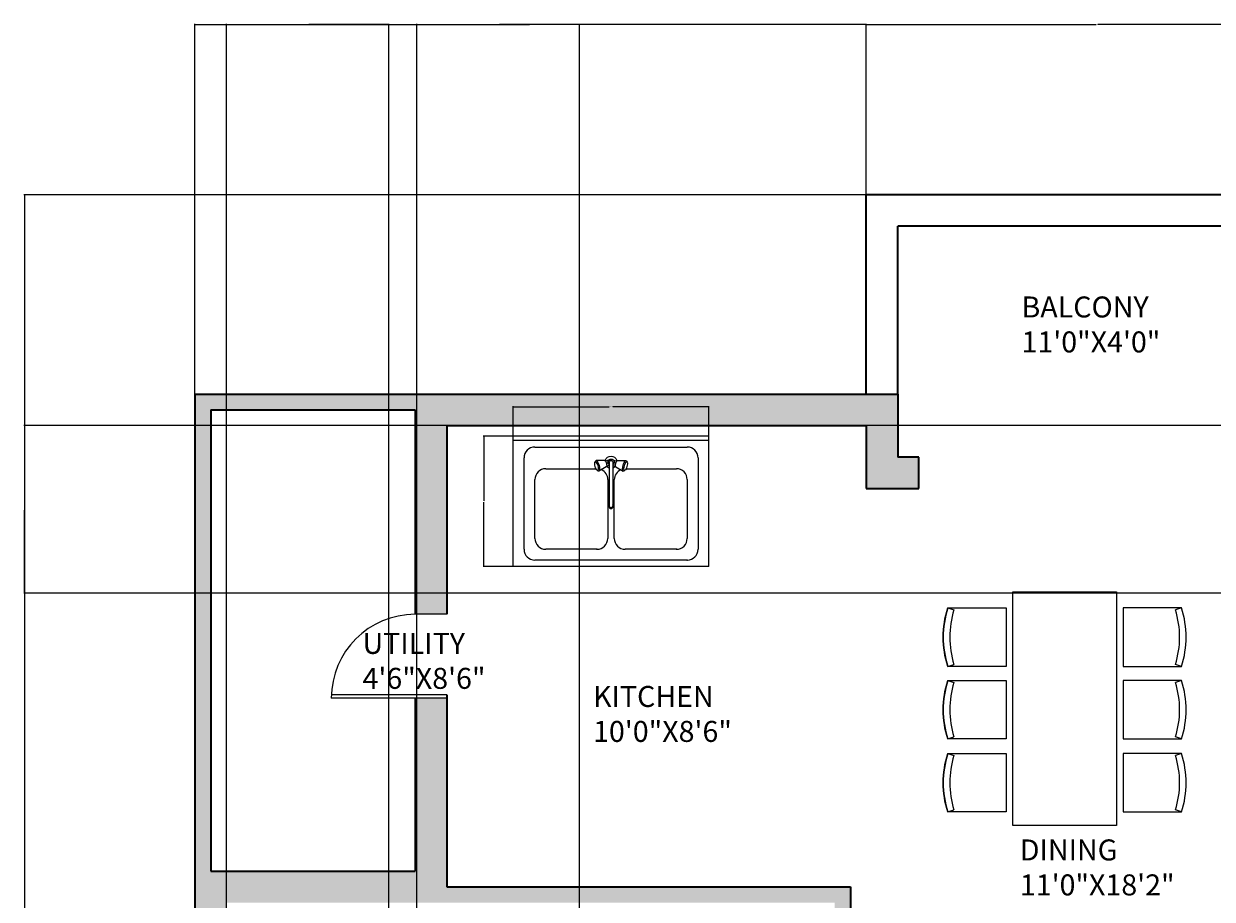
# Model space of a CAD drawing. Units: inches. Extents: x -26 to 13070, y -956 to 6917.
# Tile 8 of 13: x -26 to 314, y -134 to 116. Entities that reach past the tile are written whole.
import ezdxf

# ---------------------------------------------------------------- set-up
doc = ezdxf.new("R2010")
doc.units = ezdxf.units.IN
doc.header["$MEASUREMENT"] = 0
for name, color, linetype, lineweight in [('A-ANNO-DIMS', 2, 'Continuous', 18), ('A-AREA-IDEN', 7, 'Continuous', 18), ('A-DOOR', 3, 'Continuous', 18), ('A-FLOR-FIXT', 9, 'Continuous', 18), ('A-FURN', 8, 'Continuous', 13), ('A-WALL', 7, 'Continuous', 35), ('A-WALL-PATT', 252, 'Continuous', 13)]:
    doc.layers.add(name, color=color, linetype=linetype, lineweight=lineweight)
doc.styles.get("Standard").update_dxf_attribs({"font": 'arial.ttf'})
doc.dimstyles.get("Standard").update_dxf_attribs({"dimtxt": 0.18, "dimasz": 0.18, "dimexe": 0.18, "dimexo": 0.0625, "dimgap": 0.09, "dimtad": 0, "dimtih": 1, "dimtoh": 1, "dimdec": 0, "dimzin": 0, "dimdsep": 46, "dimlunit": 3, "dimtxsty": 'Standard', "dimcen": 0.09, "dimadec": 0, "dimazin": 0, "dimtfac": 1, "dimtdec": 0, "dimtofl": 0, "dimtmove": 0, "dimatfit": 3, "dimfxl": 1, "dimtolj": 1, "dimtzin": 0, "dimarcsym": 0})

# ---------------------------------------------------------------- blocks, each defined once
blk = doc.blocks.new('М07 600х900')
for p, q in [((0, 600), (-900, 600)), ((-900, 0), (-900, 600)), ((-900, 0), (-900, 600)), ((0, 580), (-900, 580)), ((-800, 550), (-100, 550)), ((0, 0), (0, 600)), ((0, 0), (0, 600)), ((-850, 80), (-850, 500)), ((-476.6, 488.7), (-472.7, 496.5)), ((-472.7, 496.5), (-466.5, 502.7)), ((-466.5, 502.7), (-458.7, 506.6)), ((-462.1, 488.8), (-454.6, 494.3)), ((-458.7, 506.6), (-450, 508)), ((-454.6, 494.3), (-445.4, 494.3)), ((-450, 508), (-441.3, 506.6)), ((-445.4, 494.3), (-437.9, 488.8)), ((-441.3, 506.6), (-433.5, 502.7)), ((-433.5, 502.7), (-427.3, 496.5)), ((-427.3, 496.5), (-423.4, 488.7)), ((-50, 500), (-50, 80)), ((-750, 450), (-519.1, 450)), ((-524.9, 472.1), (-524.8, 476.7)), ((-524.3, 466.5), (-524.9, 472.1)), ((-524.8, 476.7), (-523.8, 479.9)), ((-523, 460.4), (-524.3, 466.5)), ((-520.9, 485.6), (-523.8, 479.9)), ((-523.8, 479.9), (-522.2, 481.3)), ((-521.1, 454.5), (-523, 460.4)), ((-522.2, 481.3), (-520.1, 480.9)), ((-518.8, 449.4), (-521.1, 454.5)), ((-520.9, 485.6), (-518.9, 487.4)), ((-520.1, 480.9), (-517.7, 478.6)), ((-479.6, 487.6), (-518.9, 487.4)), ((-518.9, 487.4), (-516.3, 486.8)), ((-516.4, 445.5), (-518.8, 449.4)), ((-517.7, 478.6), (-515.3, 474.7)), ((-514, 443.2), (-516.4, 445.5)), ((-516.3, 486.8), (-513.3, 484)), ((-515.3, 474.7), (-513, 469.5)), ((-508.6, 439.7), (-514, 443.2)), ((-511.9, 442.7), (-514, 443.2)), ((-513.3, 484), (-510.2, 479.1)), ((-513, 469.5), (-511.1, 463.6)), ((-510.3, 444.2), (-511.9, 442.7)), ((-511.1, 463.6), (-509.8, 457.6)), ((-509.4, 447.3), (-510.3, 444.2)), ((-510.2, 479.1), (-507.4, 472.6)), ((-509.8, 457.6), (-509.2, 452)), ((-509.2, 452), (-509.4, 447.3)), ((-506, 439.1), (-508.6, 439.7)), ((-507.4, 472.6), (-505, 465.3)), ((-471.8, 458.6), (-506, 439.1)), ((-504, 440.9), (-506, 439.1)), ((-505, 465.3), (-503.4, 457.7)), ((-502.8, 444.9), (-504, 440.9)), ((-503.4, 457.7), (-502.6, 450.7)), ((-502.6, 450.7), (-502.8, 444.9)), ((-479.6, 487.6), (-478, 487.3)), ((-478, 487.3), (-476.2, 485.5)), ((-477, 486.3), (-476.6, 488.7)), ((-461.4, 489.4), (-476.2, 485.4)), ((-476.2, 485.5), (-474.4, 482.6)), ((-474.4, 482.6), (-472.7, 478.7)), ((-472.7, 478.7), (-471.2, 474.3)), ((-470.6, 459.7), (-471.8, 458.6)), ((-471.2, 474.3), (-470.3, 469.8)), ((-469.9, 462.1), (-470.6, 459.7)), ((-470.3, 469.8), (-469.8, 465.6)), ((-466.5, 457.3), (-470.2, 461.1)), ((-469.8, 465.6), (-469.9, 462.1)), ((-458.5, 465.3), (-469.9, 462.2)), ((-458.7, 453.4), (-466.5, 457.3)), ((-465, 480), (-462.1, 488.8)), ((-462.1, 471.2), (-465, 480)), ((-458.5, 468.5), (-462.1, 471.2)), ((-458.5, 453.3), (-458.7, 453.4)), ((-458.5, 480), (-456.9, 485)), ((-458.5, 480), (-458.5, 279.9)), ((-456.9, 485), (-452.6, 488.1)), ((-452.6, 488.1), (-447.4, 488.1)), ((-447.4, 488.1), (-443.1, 485)), ((-443.1, 485), (-441.5, 480)), ((-441.5, 480), (-441.5, 279.9)), ((-437.9, 471.2), (-441.5, 468.5)), ((-441.5, 465.3), (-430.1, 462.2)), ((-441.3, 453.4), (-441.5, 453.3)), ((-433.5, 457.3), (-441.3, 453.4)), ((-438.6, 489.4), (-423.8, 485.4)), ((-437.9, 488.8), (-435, 480)), ((-435, 480), (-437.9, 471.2)), ((-429.8, 461.1), (-433.5, 457.3)), ((-430.2, 465.6), (-429.7, 469.8)), ((-430.1, 462.1), (-430.2, 465.6)), ((-429.4, 459.7), (-430.1, 462.1)), ((-429.7, 469.8), (-428.8, 474.3)), ((-428.2, 458.6), (-429.4, 459.7)), ((-428.8, 474.3), (-427.3, 478.7)), ((-428.2, 458.6), (-394, 439.1)), ((-427.3, 478.7), (-425.6, 482.6)), ((-425.6, 482.6), (-423.8, 485.5)), ((-423.8, 485.5), (-422, 487.3)), ((-423.4, 488.7), (-423, 486.3)), ((-422, 487.3), (-420.4, 487.6)), ((-420.4, 487.6), (-381.1, 487.4)), ((-397.4, 450.7), (-396.6, 457.7)), ((-397.2, 444.9), (-397.4, 450.7)), ((-396, 440.9), (-397.2, 444.9)), ((-396.6, 457.7), (-395, 465.3)), ((-394, 439.1), (-396, 440.9)), ((-395, 465.3), (-392.6, 472.6)), ((-391.4, 439.7), (-394, 439.1)), ((-392.6, 472.6), (-389.8, 479.1)), ((-391.4, 439.7), (-386, 443.2)), ((-390.8, 452), (-390.2, 457.6)), ((-390.6, 447.3), (-390.8, 452)), ((-389.7, 444.2), (-390.6, 447.3)), ((-390.2, 457.6), (-388.9, 463.6)), ((-389.8, 479.1), (-386.7, 484)), ((-388.1, 442.7), (-389.7, 444.2)), ((-388.9, 463.6), (-387, 469.5)), ((-386, 443.2), (-388.1, 442.7)), ((-387, 469.5), (-384.7, 474.7)), ((-386.7, 484), (-383.7, 486.8)), ((-383.6, 445.5), (-386, 443.2)), ((-384.7, 474.7), (-382.3, 478.6)), ((-383.7, 486.8), (-381.1, 487.4)), ((-381.2, 449.4), (-383.6, 445.5)), ((-382.3, 478.6), (-379.9, 480.9)), ((-378.9, 454.5), (-381.2, 449.4)), ((-381.1, 487.4), (-379.1, 485.6)), ((-380.9, 450), (-150, 450)), ((-379.9, 480.9), (-377.8, 481.3)), ((-379.1, 485.6), (-376.2, 479.9)), ((-377, 460.4), (-378.9, 454.5)), ((-377.8, 481.3), (-376.2, 479.9)), ((-375.7, 466.5), (-377, 460.4)), ((-376.2, 479.9), (-375.2, 476.7)), ((-375.1, 472.1), (-375.7, 466.5)), ((-375.2, 476.7), (-375.1, 472.1)), ((-800, 130), (-800, 400)), ((-465, 400), (-465, 130)), ((-435, 130), (-435, 400)), ((-100, 400), (-100, 130)), ((-458.5, 285.6), (-460.5, 279.9)), ((-460.5, 279.9), (-458.5, 274.2)), ((-458.5, 279.9), (-456.9, 275.3)), ((-458.5, 274.2), (-456.9, 269.8)), ((-458.5, 274.2), (-453.2, 270.6)), ((-456.9, 275.3), (-452.6, 272.4)), ((-447.4, 272.4), (-443.1, 275.3)), ((-446.8, 270.6), (-441.5, 274.2)), ((-443.1, 275.3), (-441.5, 279.9)), ((-441.5, 274.2), (-443.1, 269.8)), ((-439.5, 279.9), (-441.5, 285.6)), ((-441.5, 274.2), (-439.5, 279.9)), ((-456.9, 269.8), (-452.6, 266.9)), ((-453.2, 270.6), (-446.8, 270.6)), ((-452.6, 272.4), (-447.4, 272.4)), ((-452.6, 266.9), (-447.4, 266.9)), ((-447.4, 266.9), (-443.1, 269.8)), ((-515, 80), (-750, 80)), ((-150, 80), (-385, 80)), ((0, 0), (-900, 0)), ((-100, 30), (-800, 30))]:
    blk.add_line(p, q)
for centre, start, end in [((-800, 500), 90, 180), ((-100, 500), 0, 90), ((-750, 400), 90, 180), ((-515, 400), 0, 65.8874), ((-385, 400), 114.1126, 180), ((-150, 400), 0, 90), ((-750, 130), 180, 270), ((-515, 130), 270, 0), ((-385, 130), 180, 270), ((-150, 130), 270, 0), ((-800, 80), 180, 270), ((-100, 80), 270, 0)]:
    blk.add_arc(centre, 50, start, end)
for p in [(-515, 80), (-150, 80), (-100, 30)]:
    blk.add_point(p)
blk = doc.blocks.new('DINING-TABLE-SIX-SEATS')
for p, q in [((1.3, 62.21), (3.07, 61.65)), ((68.16, 62.21), (66.39, 61.65)), ((1.3, 45.51), (3.07, 46.07)), ((68.16, 45.51), (66.39, 46.07)), ((1.3, 41.46), (3.07, 40.9)), ((68.16, 41.46), (66.39, 40.9)), ((1.3, 24.76), (3.07, 25.32)), ((68.16, 24.76), (66.39, 25.32)), ((1.3, 20.57), (3.07, 20.01)), ((68.16, 20.57), (66.39, 20.01)), ((1.3, 3.87), (3.07, 4.43)), ((68.16, 3.87), (66.39, 4.43))]:
    blk.add_line(p, q)
blk.add_lwpolyline([(49.58, 0), (19.88, 0), (19.88, 66.83), (49.58, 66.83)], close=True)
for points in [[(1.28, 62.21), (17.99, 62.21), (17.99, 45.51), (1.28, 45.51, -0.153703), (1.28, 62.21)], [(68.17, 62.21), (51.47, 62.21), (51.47, 45.51), (68.17, 45.51, 0.153703), (68.17, 62.21)], [(1.28, 41.46), (17.99, 41.46), (17.99, 24.76), (1.28, 24.76, -0.153703), (1.28, 41.46)], [(68.17, 41.46), (51.47, 41.46), (51.47, 24.76), (68.17, 24.76, 0.153703), (68.17, 41.46)], [(1.28, 20.57), (17.99, 20.57), (17.99, 3.87), (1.28, 3.87, -0.153703), (1.28, 20.57)], [(68.17, 20.57), (51.47, 20.57), (51.47, 3.87), (68.17, 3.87, 0.153703), (68.17, 20.57)]]:
    blk.add_lwpolyline(points, format="xyb")
for centre, radius, start, end in [((27.56, 53.86), 27.56, 162.3544, 197.6456), ((27.56, 53.86), 25.7, 162.3544, 197.6456), ((41.9, 53.86), 25.7, 342.3544, 17.6456), ((41.9, 53.86), 27.56, 342.3544, 17.6456), ((27.56, 33.11), 27.56, 162.3544, 197.6456), ((27.56, 33.11), 25.7, 162.3544, 197.6456), ((41.9, 33.11), 25.7, 342.3544, 17.6456), ((41.9, 33.11), 27.56, 342.3544, 17.6456), ((27.56, 12.22), 27.56, 162.3544, 197.6456), ((41.9, 12.22), 27.56, 342.3544, 17.6456), ((27.56, 12.22), 25.7, 162.3544, 197.6456), ((41.9, 12.22), 25.7, 342.3544, 17.6456)]:
    blk.add_arc(centre, radius, start, end)
blk = doc.blocks.new('DOOR-SWING-24')
for p, q in [((24, 1), (0, 1)), ((24, 0), (0, 0))]:
    blk.add_line(p, q)
blk.add_arc((24, 0), 24, 90, 180)
blk = doc.blocks.new('*D32')
at = {"layer": 'A-ANNO-DIMS', "color": 0, "lineweight": -2, "transparency": 16777216}
for p, q in [((113.65, -1.51), (113.65, 7.01)), ((113.83, 6.83), (141.11, 6.83)), ((169.48, 6.83), (142.2, 6.83)), ((169.66, -1.51), (169.66, 7.01))]:
    blk.add_line(p, q, dxfattribs=at)
at = {"layer": 'A-ANNO-DIMS', "color": 0, "transparency": 16777216}
for points in [[(113.83, 6.86), (113.83, 6.8), (113.65, 6.83)], [(169.48, 6.86), (169.48, 6.8), (169.66, 6.83)]]:
    blk.add_solid(points, dxfattribs=at)
at = {"layer": 'Defpoints', "color": 0, "transparency": 16777216}
for p in [(169.66, 6.83), (113.65, -1.57), (169.66, -1.57)]:
    blk.add_point(p, dxfattribs=at)
at = {"layer": 'A-ANNO-DIMS', "color": 0, "transparency": 16777216, "insert": (141.66, 6.83), "char_height": 0.18, "attachment_point": 5}
blk.add_mtext('\\A1;SINK 56', dxfattribs=at)
blk = doc.blocks.new('*D33')
at = {"layer": 'A-ANNO-DIMS', "color": 0, "lineweight": -2, "transparency": 16777216}
for p, q in [((113.59, -1.57), (105.07, -1.57)), ((105.25, -1.75), (105.25, -20.06)), ((105.25, -38.73), (105.25, -20.42)), ((113.59, -38.91), (105.07, -38.91))]:
    blk.add_line(p, q, dxfattribs=at)
at = {"layer": 'A-ANNO-DIMS', "color": 0, "transparency": 16777216}
for points in [[(105.22, -1.75), (105.28, -1.75), (105.25, -1.57)], [(105.22, -38.73), (105.28, -38.73), (105.25, -38.91)]]:
    blk.add_solid(points, dxfattribs=at)
at = {"layer": 'Defpoints', "color": 0, "transparency": 16777216}
for p in [(105.25, -1.57), (113.65, -1.57), (113.65, -38.91)]:
    blk.add_point(p, dxfattribs=at)
at = {"layer": 'A-ANNO-DIMS', "color": 0, "transparency": 16777216, "insert": (105.25, -20.24), "char_height": 0.18, "attachment_point": 5}
blk.add_mtext('\\A1;37', dxfattribs=at)
blk = doc.blocks.new('*D41')
at = {"layer": 'A-ANNO-DIMS', "color": 0, "lineweight": -2, "transparency": 16777216}
for p, q in [((214.58, 67.46), (-26.29, 67.46)), ((-26.11, 67.28), (-26.11, -419.86)), ((-26.11, -907.36), (-26.11, -420.22)), ((208.58, -907.54), (-26.29, -907.54))]:
    blk.add_line(p, q, dxfattribs=at)
at = {"layer": 'A-ANNO-DIMS', "color": 0, "transparency": 16777216}
for points in [[(-26.14, 67.28), (-26.08, 67.28), (-26.11, 67.46)], [(-26.14, -907.36), (-26.08, -907.36), (-26.11, -907.54)]]:
    blk.add_solid(points, dxfattribs=at)
at = {"layer": 'Defpoints', "color": 0, "transparency": 16777216}
for p in [(-26.11, 67.46), (214.64, 67.46), (208.64, -907.54)]:
    blk.add_point(p, dxfattribs=at)
at = {"layer": 'A-ANNO-DIMS', "color": 0, "transparency": 16777216, "insert": (-26.11, -420.04), "char_height": 0.18, "attachment_point": 5}
blk.add_mtext('\\A1;975', dxfattribs=at)
blk = doc.blocks.new('*D42')
at = {"layer": 'A-ANNO-DIMS', "color": 0, "lineweight": -2, "transparency": 16777216}
for p, q in [((22.64, 10.52), (22.64, 116.39)), ((22.82, 116.21), (118.36, 116.21)), ((214.46, 116.21), (118.92, 116.21)), ((214.64, 67.52), (214.64, 116.39))]:
    blk.add_line(p, q, dxfattribs=at)
at = {"layer": 'A-ANNO-DIMS', "color": 0, "transparency": 16777216}
for points in [[(22.82, 116.24), (22.82, 116.18), (22.64, 116.21)], [(214.46, 116.24), (214.46, 116.18), (214.64, 116.21)]]:
    blk.add_solid(points, dxfattribs=at)
at = {"layer": 'Defpoints', "color": 0, "transparency": 16777216}
for p in [(214.64, 116.21), (214.64, 67.46), (22.64, 10.46)]:
    blk.add_point(p, dxfattribs=at)
at = {"layer": 'A-ANNO-DIMS', "color": 0, "transparency": 16777216, "insert": (118.64, 116.21), "char_height": 0.18, "attachment_point": 5}
blk.add_mtext('\\A1;192', dxfattribs=at)
blk = doc.blocks.new('*D43')
at = {"layer": 'A-ANNO-DIMS', "color": 0, "lineweight": -2, "transparency": 16777216}
for p, q in [((214.64, 67.52), (214.64, 116.39)), ((214.82, 116.21), (280.36, 116.21)), ((346.46, 116.21), (280.92, 116.21)), ((346.64, 67.52), (346.64, 116.39))]:
    blk.add_line(p, q, dxfattribs=at)
at = {"layer": 'A-ANNO-DIMS', "color": 0, "transparency": 16777216}
for points in [[(214.82, 116.24), (214.82, 116.18), (214.64, 116.21)], [(346.46, 116.24), (346.46, 116.18), (346.64, 116.21)]]:
    blk.add_solid(points, dxfattribs=at)
at = {"layer": 'Defpoints', "color": 0, "transparency": 16777216}
for p in [(346.64, 116.21), (214.64, 67.46), (346.64, 67.46)]:
    blk.add_point(p, dxfattribs=at)
at = {"layer": 'A-ANNO-DIMS', "color": 0, "transparency": 16777216, "insert": (280.64, 116.21), "char_height": 0.18, "attachment_point": 5}
blk.add_mtext('\\A1;132', dxfattribs=at)
blk = doc.blocks.new('*D55')
at = {"layer": 'A-ANNO-DIMS', "color": 0, "lineweight": -2, "transparency": 16777216}
for p, q in [((31.64, -327.23), (31.64, 116.39)), ((31.82, 116.21), (54.56, 116.21)), ((77.96, 116.21), (55.22, 116.21)), ((78.14, -327.23), (78.14, 116.39))]:
    blk.add_line(p, q, dxfattribs=at)
at = {"layer": 'A-ANNO-DIMS', "color": 0, "transparency": 16777216}
for points in [[(31.82, 116.24), (31.82, 116.18), (31.64, 116.21)], [(77.96, 116.24), (77.96, 116.18), (78.14, 116.21)]]:
    blk.add_solid(points, dxfattribs=at)
at = {"layer": 'Defpoints', "color": 0, "transparency": 16777216}
for p in [(78.14, 116.21), (31.64, -327.29), (78.14, -327.29)]:
    blk.add_point(p, dxfattribs=at)
at = {"layer": 'A-ANNO-DIMS', "color": 0, "transparency": 16777216, "insert": (54.89, 116.21), "char_height": 0.18, "attachment_point": 5}
blk.add_mtext('\\A1;46.5', dxfattribs=at)
blk = doc.blocks.new('*D56')
at = {"layer": 'A-ANNO-DIMS', "color": 0, "lineweight": -2, "transparency": 16777216}
for p, q in [((86.14, -327.23), (86.14, 116.39)), ((86.32, 116.21), (109.06, 116.21)), ((132.46, 116.21), (109.72, 116.21)), ((132.64, -327.23), (132.64, 116.39))]:
    blk.add_line(p, q, dxfattribs=at)
at = {"layer": 'A-ANNO-DIMS', "color": 0, "transparency": 16777216}
for points in [[(86.32, 116.24), (86.32, 116.18), (86.14, 116.21)], [(132.46, 116.24), (132.46, 116.18), (132.64, 116.21)]]:
    blk.add_solid(points, dxfattribs=at)
at = {"layer": 'Defpoints', "color": 0, "transparency": 16777216}
for p in [(132.64, 116.21), (86.14, -327.29), (132.64, -327.29)]:
    blk.add_point(p, dxfattribs=at)
at = {"layer": 'A-ANNO-DIMS', "color": 0, "transparency": 16777216, "insert": (109.39, 116.21), "char_height": 0.18, "attachment_point": 5}
blk.add_mtext('\\A1;46.5', dxfattribs=at)
blk = doc.blocks.new('*D58')
at = {"layer": 'A-ANNO-DIMS', "color": 0, "lineweight": -2, "transparency": 16777216}
for p, q in [((538.58, 1.46), (-26.29, 1.46)), ((-26.11, 1.28), (-26.11, -22.36)), ((-26.11, -46.36), (-26.11, -22.72)), ((538.58, -46.54), (-26.29, -46.54))]:
    blk.add_line(p, q, dxfattribs=at)
at = {"layer": 'A-ANNO-DIMS', "color": 0, "transparency": 16777216}
for points in [[(-26.14, 1.28), (-26.08, 1.28), (-26.11, 1.46)], [(-26.14, -46.36), (-26.08, -46.36), (-26.11, -46.54)]]:
    blk.add_solid(points, dxfattribs=at)
at = {"layer": 'Defpoints', "color": 0, "transparency": 16777216}
for p in [(-26.11, 1.46), (538.64, 1.46), (538.64, -46.54)]:
    blk.add_point(p, dxfattribs=at)
at = {"layer": 'A-ANNO-DIMS', "color": 0, "transparency": 16777216, "insert": (-26.11, -22.54), "char_height": 0.18, "attachment_point": 5}
blk.add_mtext('\\A1;48', dxfattribs=at)

msp = doc.modelspace()

# ---------------------------------------------------------------- hatches: boundary and pattern name
at = {"layer": 'A-WALL-PATT'}
h = msp.add_hatch(color=256, dxfattribs=at)
h.dxf.hatch_style = 1
h.paths.add_polyline_path([(223.641, 10.458), (214.641, 10.458), (22.641, 10.458), (22.641, -171.042), (31.641, -171.042), (31.641, -135.042), (205.641, -135.042), (205.641, -241.042), (210.141, -241.042), (210.141, -130.542), (94.641, -130.542), (94.641, -76.542), (85.641, -76.542), (85.641, -126.042), (27.141, -126.042), (27.141, 5.958), (85.641, 5.958), (85.641, -52.542), (94.641, -52.542), (94.641, 1.458), (214.641, 1.458), (214.641, -16.542), (223.641, -16.542), (229.641, -16.542), (229.641, -7.542), (223.641, -7.542)])
h.paths.add_polyline_path([(367.048, 10.458), (346.641, 10.458), (337.641, 10.458), (337.641, -7.542), (331.641, -7.542), (331.641, -16.542), (337.641, -16.542), (342.141, -16.542), (342.141, -128.542), (346.641, -128.542), (346.641, 1.458), (367.048, 1.458)])
h.paths.add_polyline_path([(547.641, 10.458), (403.048, 10.458), (403.048, 1.458), (538.641, 1.458), (538.641, -46.542), (547.641, -46.542)])
h.paths.add_polyline_path([(547.641, -106.542), (538.641, -106.542), (538.641, -154.542), (481.013, -154.542), (481.013, -159.042), (538.641, -159.042), (547.641, -159.042)])
h.paths.add_polyline_path([(457.013, -154.542), (342.141, -154.542), (342.141, -165.042), (346.641, -165.042), (346.641, -159.042), (414.141, -159.042), (414.141, -225.042), (346.641, -225.042), (346.641, -189.042), (342.141, -189.042), (342.141, -234.042), (390.641, -234.042), (390.641, -286.042), (395.141, -286.042), (395.141, -234.042), (456.141, -234.042), (456.141, -312.042), (372.641, -312.042), (372.641, -316.542), (462.641, -316.542), (462.641, -312.042), (460.641, -312.042), (460.641, -234.042), (538.641, -234.042), (547.641, -234.042), (547.641, -195.042), (538.641, -195.042), (538.641, -225.042), (418.641, -225.042), (418.641, -159.042), (457.013, -159.042)])
h.paths.add_polyline_path([(547.641, -270.042), (538.641, -270.042), (538.641, -312.042), (486.641, -312.042), (486.641, -316.542), (538.641, -316.542), (547.641, -316.542)], flags=0)
h.paths.add_polyline_path([(547.641, -456.306), (538.641, -456.306), (538.641, -457.542), (346.641, -457.542), (346.641, -316.542), (346.641, -312.042), (342.141, -312.042), (342.141, -457.542), (145.641, -457.542), (145.641, -466.542), (342.141, -466.542), (342.141, -627.042), (346.641, -627.042), (346.641, -466.542), (538.641, -466.542), (538.641, -514.542), (547.641, -514.542)])
h.paths.add_polyline_path([(466.641, -622.542), (372.641, -622.542), (372.641, -627.042), (388.641, -627.042), (388.641, -721.542), (393.141, -721.542), (393.141, -627.042), (462.141, -627.042), (462.141, -717.042), (466.641, -717.042)])
h.paths.add_polyline_path([(547.641, -574.542), (538.641, -574.542), (538.641, -622.542), (492.641, -622.542), (492.641, -627.042), (538.641, -627.042), (538.641, -654.042), (547.641, -654.042)])
h.paths.add_polyline_path([(547.641, -690.042), (538.641, -690.042), (538.641, -717.042), (466.641, -717.042), (466.641, -721.542), (538.641, -721.542), (538.641, -763.542), (547.641, -763.542)])
h.paths.add_polyline_path([(462.141, -717.042), (419.141, -717.042), (419.141, -721.542), (462.141, -721.542)], flags=0)
h.paths.add_polyline_path([(346.641, -721.542), (352.641, -721.542), (352.641, -717.042), (342.141, -717.042), (342.141, -874.542), (342.141, -907.542), (351.141, -907.542), (351.141, -874.542), (395.949, -874.542), (395.949, -865.542), (351.141, -865.542), (351.141, -841.542), (346.641, -841.542)])
h.paths.add_polyline_path([(547.641, -823.542), (538.641, -823.542), (538.641, -865.542), (431.949, -865.542), (431.949, -874.542), (547.641, -874.542)])
h.paths.add_polyline_path([(172.641, -865.713), (140.641, -865.744), (140.641, -788.744), (182.646, -788.704), (182.641, -784.204), (136.141, -784.249), (136.141, -848.332), (131.641, -848.332), (131.641, -874.542), (172.641, -874.542)])
h.paths.add_polyline_path([(217.641, -816.13), (213.141, -816.13), (213.141, -784.174), (208.641, -784.179), (208.641, -865.679), (208.641, -874.542), (217.641, -874.542)])
h.paths.add_polyline_path([(95.641, -865.788), (31.641, -865.849), (31.641, -832.695), (22.641, -832.695), (22.641, -874.542), (95.641, -874.542)])
h.paths.add_polyline_path([(217.641, -741.17), (31.641, -741.349), (31.641, -708.349), (22.641, -708.349), (22.641, -772.542), (22.641, -796.695), (31.641, -796.695), (31.641, -763.542), (31.641, -745.849), (217.641, -745.67)])
h.paths.add_polyline_path([(31.641, -651.349), (99.65, -651.284), (99.641, -642.284), (31.641, -642.349), (31.641, -639.042), (31.641, -588.349), (125.641, -588.259), (125.641, -651.259), (134.641, -651.25), (134.641, -579.25), (112.641, -579.271), (112.641, -549.042), (112.641, -504.271), (85.633, -504.297), (85.641, -513.297), (103.641, -513.28), (103.641, -549.042), (103.641, -579.28), (31.641, -579.349), (31.641, -549.042), (31.641, -513.349), (49.641, -513.314), (49.633, -504.332), (31.641, -504.349), (22.641, -504.358), (22.641, -684.349), (31.641, -684.349)])
h.paths.add_polyline_path([(31.641, -276.042), (145.641, -276.042), (145.641, -402.042), (145.641, -419.542), (154.641, -419.542), (154.641, -411.042), (154.641, -271.542), (210.141, -271.542), (210.141, -265.042), (205.641, -265.042), (205.641, -267.042), (31.641, -267.042), (31.641, -231.042), (22.641, -231.042), (22.641, -426.852), (31.641, -426.852), (31.641, -411.042), (31.641, -402.042)])

# ---------------------------------------------------------------- linework, layer by layer
at = {"layer": 'A-DOOR'}
for p, q in [((94.641, -52.542), (85.641, -52.542)), ((94.641, -75.542), (85.641, -75.542)), ((94.641, -76.542), (85.641, -76.542))]:
    msp.add_line(p, q, dxfattribs=at)
at = {"layer": 'A-WALL'}
for p, q in [((214.641, 10.458), (214.641, 67.458)), ((337.641, 67.458), (214.641, 67.458)), ((337.641, 58.458), (223.641, 58.458)), ((223.641, 10.458), (223.641, 58.458)), ((22.641, 10.458), (22.641, -772.542)), ((22.641, 10.458), (214.641, 10.458)), ((214.641, 10.458), (223.641, 10.458)), ((223.641, 10.458), (223.641, -7.542)), ((27.141, 5.958), (27.141, -126.042)), ((27.141, 5.958), (85.641, 5.958)), ((85.641, 5.958), (85.641, -52.542)), ((94.641, 1.458), (214.641, 1.458)), ((94.641, 1.458), (94.641, -52.542)), ((214.641, 1.458), (214.641, -16.542)), ((229.641, -7.542), (223.641, -7.542)), ((229.641, -16.542), (229.641, -7.542)), ((214.641, -16.542), (223.641, -16.542)), ((223.641, -16.542), (229.641, -16.542)), ((85.641, -76.542), (85.641, -126.042)), ((94.641, -75.542), (94.641, -130.542)), ((27.141, -126.042), (85.641, -126.042)), ((94.641, -130.542), (210.141, -130.542)), ((210.141, -130.542), (210.141, -241.042))]:
    msp.add_line(p, q, dxfattribs=at)

# ---------------------------------------------------------------- block references
at = {"layer": 'A-DOOR'}
msp.add_blockref('DOOR-SWING-24', (61.641, -76.542), dxfattribs=at)
at = {"layer": 'A-FLOR-FIXT', "xscale": 0.0622343831229516, "yscale": 0.0622343831229516, "zscale": 0.0622343831229516}
msp.add_blockref('М07 600х900', (169.661, -38.911), dxfattribs=at)
at = {"layer": 'A-FURN'}
msp.add_blockref('DINING-TABLE-SIX-SEATS', (236.665, -112.945), dxfattribs=at)

# ---------------------------------------------------------------- texts
at = {"layer": 'A-AREA-IDEN', "char_height": 6, "attachment_point": 1}
for s, insert in [('BALCONY\\P11\'0"X4\'0"', (259.048, 38.373)), ('UTILITY\\P4\'6"X8\'6"', (70.574, -57.86)), ('KITCHEN\\P10\'0"X8\'6"', (136.506, -73.043))]:
    msp.add_mtext(s, dxfattribs=dict(at, insert=insert))
at = {"layer": 'A-AREA-IDEN', "insert": (258.573, -116.944), "char_height": 6, "attachment_point": 1}
msp.add_mtext_dynamic_manual_height_columns('DINING\\P11\'0"X18\'2"', width=0.33656, gutter_width=1, heights=[0], dxfattribs=at)

# ---------------------------------------------------------------- dimensions: what is measured, and where the dimension line sits
at = {"layer": 'A-ANNO-DIMS'}
for base, p1, p2, override, picture, middle in [((214.641, 116.209), (22.641, 10.458), (214.641, 67.458), {"dimdec": 0, "dimlfac": 1, "dimrnd": 0, "dimzin": 0, "dimdsep": 46, "dimlunit": 2}, '*D42', (118.641, 116.209)), ((78.141, 116.209), (31.641, -327.292), (78.141, -327.292), {"dimdec": 1, "dimlfac": 1, "dimrnd": 0, "dimzin": 0, "dimdsep": 46, "dimlunit": 2}, '*D55', (54.891, 116.209)), ((132.641, 116.209), (86.141, -327.292), (132.641, -327.292), {"dimdec": 1, "dimlfac": 1, "dimrnd": 0, "dimzin": 0, "dimdsep": 46, "dimlunit": 2}, '*D56', (109.391, 116.209)), ((346.641, 116.209), (214.641, 67.458), (346.641, 67.458), {"dimdec": 0, "dimlfac": 1, "dimrnd": 0, "dimzin": 0, "dimdsep": 46, "dimlunit": 2}, '*D43', (280.641, 116.209))]:
    dim = msp.add_linear_dim(base=base, p1=p1, p2=p2, dimstyle='Standard', override=override, dxfattribs=at)
    dim.commit()
    dim.dimension.update_dxf_attribs({"geometry": picture, "text_midpoint": middle})
for base, p1, p2, picture, middle in [((-26.11, 67.458), (208.641, -907.542), (214.641, 67.458), '*D41', (-26.11, -420.042)), ((-26.11, 1.458), (538.641, -46.542), (538.641, 1.458), '*D58', (-26.11, -22.542)), ((105.249, -1.57), (113.65, -38.911), (113.65, -1.57), '*D33', (105.249, -20.241))]:
    dim = msp.add_linear_dim(base=base, p1=p1, p2=p2, angle=90, dimstyle='Standard', override={"dimdec": 0, "dimlfac": 1, "dimrnd": 0, "dimzin": 0, "dimdsep": 46, "dimlunit": 2}, dxfattribs=at)
    dim.commit()
    dim.dimension.update_dxf_attribs({"geometry": picture, "text_midpoint": middle})
dim = msp.add_linear_dim(base=(169.661, 6.831), p1=(113.65, -1.57), p2=(169.661, -1.57), text='SINK <>', dimstyle='Standard', override={"dimdec": 0, "dimlfac": 1, "dimrnd": 0, "dimzin": 0, "dimdsep": 46, "dimlunit": 2}, dxfattribs=at)
dim.commit()
dim.dimension.update_dxf_attribs({"geometry": '*D32', "text_midpoint": (141.656, 6.831)})

doc.saveas('drawing.dxf')
